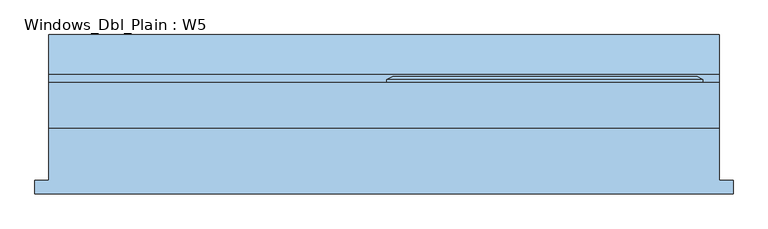
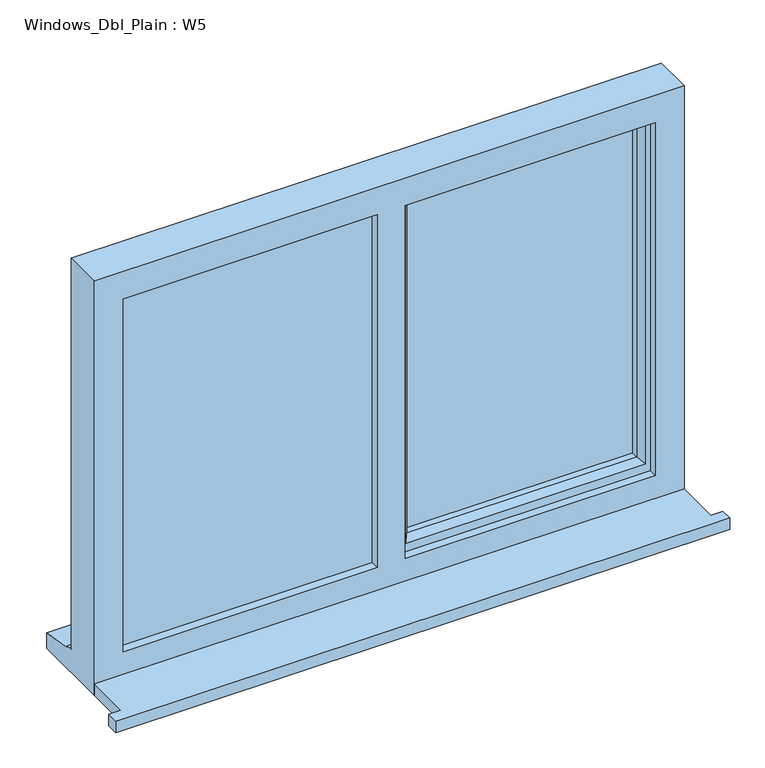
"""IFC4 building model written with IfcOpenShell, lengths in millimetres: window geometry, Windows_Dbl_Plain : W5."""

from ifc_helpers import new_model, si_unit, frame, origin, place, context, project, spatial, polyline, outline, extrude, faceted_brep, source, transform, mapped, element, save


def windows_dbl_plain_w5_c0a8d941(model_context):
    return source(origin(), model_context, "Body", "SolidModel", [
        extrude(outline(polyline([(-922.3432, -130.8434322), (-922.3432, -105.8434322), (-897.3432, -105.8434322), (-897.3432, -10.2434322), (327.3432, -10.2434322), (327.3432, -105.8434322), (352.3432, -105.8434322), (352.3432, -130.8434322), (-922.3432, -130.8434322)])), frame((0.0, 0.0, 1200.0), z_axis=(0.0, 0.0, 1.0), x_axis=(1.0, 0.0, 0.0)), (0.0, 0.0, 1.0), 25.0),
        faceted_brep([(-280.0, 72.7565678, 2080.0), (-280.0, 78.5300705, 2080.0), (-280.0, 78.5300705, 1253.0), (-280.0, 72.7565678, 1253.0), (-270.0, 7.7565678, 2070.0), (-270.0, 72.7565678, 2070.0), (-270.0, 72.7565678, 1263.0), (-270.0, 7.7565678, 1263.0), (-230.0, 22.2494677, 2030.0), (-240.1480377, 7.7565678, 2040.1480377), (-240.1480377, 7.7565678, 1292.8519623), (-230.0, 22.2494677, 1303.0), (-230.0, 36.7565678, 2030.0), (-230.0, 36.7565678, 1303.0), (-240.0, 60.7565678, 2040.0), (-240.0, 36.7565678, 2040.0), (-240.0, 36.7565678, 1293.0), (-240.0, 60.7565678, 1293.0), (-230.0, 78.5300705, 2030.0), (-230.0, 60.7565678, 2030.0), (-230.0, 60.7565678, 1303.0), (-230.0, 78.5300705, 1303.0), (-247.4457548, 84.3035732, 2047.4457548), (-247.4457548, 84.3035732, 1285.5542452), (-269.2153903, 84.3035732, 2069.2153903), (-269.2153903, 84.3035732, 1263.7846097), (297.3432, 78.5300705, 1253.0), (297.3432, 72.7565678, 1253.0), (287.3432, 72.7565678, 1263.0), (287.3432, 7.7565678, 1263.0), (257.4912377, 7.7565678, 1292.8519623), (247.3432, 22.2494677, 1303.0), (247.3432, 36.7565678, 1303.0), (257.3432, 36.7565678, 1293.0), (257.3432, 60.7565678, 1293.0), (247.3432, 60.7565678, 1303.0), (247.3432, 78.5300705, 1303.0), (264.7889548, 84.3035732, 1285.5542452), (286.5585903, 84.3035732, 1263.7846097), (297.3432, 78.5300705, 2080.0), (297.3432, 72.7565678, 2080.0), (287.3432, 72.7565678, 2070.0), (287.3432, 7.7565678, 2070.0), (257.4912377, 7.7565678, 2040.1480377), (247.3432, 22.2494677, 2030.0), (247.3432, 36.7565678, 2030.0), (257.3432, 36.7565678, 2040.0), (257.3432, 60.7565678, 2040.0), (247.3432, 60.7565678, 2030.0), (247.3432, 78.5300705, 2030.0), (264.7889548, 84.3035732, 2047.4457548), (286.5585903, 84.3035732, 2069.2153903)], [[[0, 1, 2, 3]], [[4, 5, 6, 7]], [[8, 9, 10, 11]], [[12, 8, 11, 13]], [[14, 15, 16, 17]], [[18, 19, 20, 21]], [[22, 18, 21, 23]], [[1, 24, 25, 2]], [[3, 2, 26, 27]], [[7, 6, 28, 29]], [[11, 10, 30, 31]], [[13, 11, 31, 32]], [[17, 16, 33, 34]], [[21, 20, 35, 36]], [[23, 21, 36, 37]], [[2, 25, 38, 26]], [[27, 26, 39, 40]], [[29, 28, 41, 42]], [[31, 30, 43, 44]], [[32, 31, 44, 45]], [[34, 33, 46, 47]], [[36, 35, 48, 49]], [[37, 36, 49, 50]], [[26, 38, 51, 39]], [[40, 39, 1, 0]], [[3, 27, 40, 0], [5, 41, 28, 6]], [[42, 41, 5, 4]], [[7, 29, 42, 4], [9, 43, 30, 10]], [[44, 43, 9, 8]], [[45, 44, 8, 12]], [[15, 46, 33, 16], [13, 32, 45, 12]], [[47, 46, 15, 14]], [[17, 34, 47, 14], [19, 48, 35, 20]], [[49, 48, 19, 18]], [[50, 49, 18, 22]], [[24, 51, 38, 25], [23, 37, 50, 22]], [[39, 51, 24, 1]]]),
        extrude(outline(polyline([(2050.0, -310.0), (2070.0, -310.0), (2070.0, -857.3432), (1263.0, -857.3432), (1263.0, -310.0), (1283.0, -310.0), (1283.0, -837.3432), (2050.0, -837.3432), (2050.0, -310.0)])), frame((0.0, 31.7565678, 0.0), z_axis=(0.0, 1.0, 0.0), x_axis=(0.0, 0.0, 1.0)), (0.0, 0.0, 1.0), 41.0),
        faceted_brep([(327.3432, -10.2434322, 2110.0), (-897.3432, -10.2434322, 2110.0), (-897.3432, -10.2434322, 1200.0), (327.3432, -10.2434322, 1200.0), (267.3432, -10.2434322, 2050.0), (267.3432, -10.2434322, 1275.0), (-252.0, -10.2434322, 1275.0), (-252.0, -10.2434322, 2050.0), (-310.0, -10.2434322, 2050.0), (-310.0, -10.2434322, 1275.0), (-837.3432, -10.2434322, 1275.0), (-837.3432, -10.2434322, 2050.0), (-897.3432, 72.7565678, 2110.0), (-897.3432, 72.7565678, 1251.0), (-897.3432, 87.7565678, 1249.68767), (-897.3432, 87.7565678, 1244.7449676), (-897.3432, 160.2565678, 1233.8088847), (-897.3432, 160.2565678, 1200.0), (327.3432, 72.7565678, 2110.0), (327.3432, 72.7565678, 1251.0), (-857.3432, 72.7565678, 2070.0), (-857.3432, 72.7565678, 1263.0), (-310.0, 72.7565678, 1263.0), (-310.0, 72.7565678, 2070.0), (-270.0, 72.7565678, 2070.0), (-270.0, 72.7565678, 1263.0), (287.3432, 72.7565678, 1263.0), (287.3432, 72.7565678, 2070.0), (-857.3432, 7.7565678, 2070.0), (-857.3432, 7.7565678, 1263.0), (-300.0, 7.7565678, 2070.0), (-300.0, 7.7565678, 1263.0), (-310.0, 7.7565678, 2050.0), (-837.3432, 7.7565678, 2050.0), (-837.3432, 7.7565678, 1275.0), (-310.0, 7.7565678, 1275.0), (-270.0, 7.7565678, 2070.0), (287.3432, 7.7565678, 2070.0), (287.3432, 7.7565678, 1263.0), (-270.0, 7.7565678, 1263.0), (267.3432, 7.7565678, 2050.0), (-252.0, 7.7565678, 2050.0), (-252.0, 7.7565678, 1275.0), (267.3432, 7.7565678, 1275.0), (-310.0, 31.7565678, 2070.0), (-300.0, 31.7565678, 2070.0), (327.3432, 160.2565678, 1200.0), (327.3432, 160.2565678, 1233.8088847), (327.3432, 87.7565678, 1244.7449676), (327.3432, 87.7565678, 1249.68767), (-300.0, 31.7565678, 1263.0), (-310.0, 31.7565678, 1263.0)], [[[0, 1, 2, 3], [4, 5, 6, 7], [8, 9, 10, 11]], [[2, 1, 12, 13, 14, 15, 16, 17]], [[13, 12, 18, 19], [20, 21, 22, 23], [24, 25, 26, 27]], [[21, 20, 28, 29]], [[28, 30, 31, 29], [32, 33, 34, 35]], [[36, 37, 38, 39], [40, 41, 42, 43]], [[33, 11, 10, 34]], [[1, 0, 18, 12]], [[28, 20, 23, 44, 45, 30]], [[27, 37, 36, 24]], [[11, 33, 32, 8]], [[40, 4, 7, 41]], [[19, 18, 0, 3, 46, 47, 48, 49]], [[27, 26, 38, 37]], [[4, 40, 43, 5]], [[45, 50, 31, 30]], [[50, 45, 44, 51]], [[51, 44, 23, 22]], [[25, 24, 36, 39]], [[41, 7, 6, 42]], [[8, 32, 35, 9]], [[46, 3, 2, 17]], [[47, 46, 17, 16]], [[48, 47, 16, 15]], [[49, 48, 15, 14]], [[19, 49, 14, 13]], [[22, 21, 29, 31, 50, 51]], [[26, 25, 39, 38]], [[6, 5, 43, 42]], [[35, 34, 10, 9]]]),
        extrude(outline(polyline([(-857.3432, 31.7565678), (-300.0, 31.7565678), (-300.0, 7.7565678), (-857.3432, 7.7565678), (-857.3432, 31.7565678)])), frame((0.0, 0.0, 1263.0), z_axis=(0.0, 0.0, 1.0), x_axis=(1.0, 0.0, 0.0)), (0.0, 0.0, 1.0), 807.0),
        extrude(outline(polyline([(257.3432, 36.7565678), (-240.0, 36.7565678), (-240.0, 60.7565678), (257.3432, 60.7565678), (257.3432, 36.7565678)])), frame((0.0, 0.0, 1293.0), z_axis=(0.0, 0.0, 1.0), x_axis=(1.0, 0.0, 0.0)), (0.0, 0.0, 1.0), 747.0),
    ])


if __name__ == "__main__":
    model = new_model("IFC4")
    model_context = context("Model", 3, world=origin())
    ifc_project = project(units=[si_unit("LENGTHUNIT", "METRE", prefix="MILLI")], contexts=[model_context])
    site = spatial("IfcSite", under=ifc_project)
    building = spatial("IfcBuilding", under=site)
    placement = place(None, origin())
    windows_dbl_plain_w5_shape = windows_dbl_plain_w5_c0a8d941(model_context)
    element("IfcWindow", 1, ObjectType="Windows_Dbl_Plain : W5", at=placement, inside=building, context=model_context, shape_type="MappedRepresentation", body=[
        mapped(windows_dbl_plain_w5_shape, transform((0.0, 0.0, 0.0), x_axis=(1.0, 0.0, 0.0), y_axis=(0.0, 1.0, 0.0), z_axis=(0.0, 0.0, 1.0))),
    ])
    save(model, "model.ifc")

# Revit data of these elements
# Type "Windows_Dbl_Plain : W5"
#   Type Mark = "57"
#   Operation = "DoublePanelVertical"
#   Construction Type Id = "GSP4R"
#   Manufacturer = "Revit"
#   Keynote = "L10"
#   Analytic Construction = "1/8 in Pilkington single glazing"
#   Wrap Layers (Ext) from Ext = 0.336286 ft
#   Wrap Layers (Int) from Ext = 0.582349 ft
#   Window Board Projection = 0.082021 ft
#   Window Board Extension = 0.082021 ft
#   Visual Light Transmittance = 0.9
#   Solar Heat Gain Coefficient = 0.78
#   Rough Width = 4.018 ft
#   Rough Height = 2.985564 ft
#   Height = 2.985564 ft
#   Width = 4.018 ft
#   Heat Transfer Coefficient (U) = 3.6886 W/(m²·K)
#   Glazing Thickness = 0.07874 ft
#   FrameOffset - External = 0.164042 ft
#   Frame Depth = 0.213255 ft
#   Default Head Height = 6.922572 ft
#   Cill Depth = 0.287073 ft
#   Cavity Closer Width = 0.164042 ft
#   Cavity Closer Offset from Ext = 0.336286 ft
#   Cavity Closer Depth = 0.278871 ft
#   Vis - Cavity Closers = yes
#   Define Thermal Properties by = 1
#   Material Trim = Window Frame
#   Material Glass = Glass
#   Material Frame = Cherry
#   Wall Closure = (empty or 0)
# Element 1 (IfcWindow, "Windows_Dbl_Plain : W5")
#   Materials on its faces: "Cherry", "Glass", "Window Frame"
# Materials
#   "Window Frame": colour RGB 249 249 249, transparency 0, Keynote = "L10", Cost = 0
#   "Glass": class "Glass", colour RGB 0 128 192, transparency 0.9, Description = "Soda Lime Glass", Cost = 0
#   "Cherry": class "Wood", colour RGB 226 177 128, transparency 0, Description = "Prunus Serotina", Cost = 0
